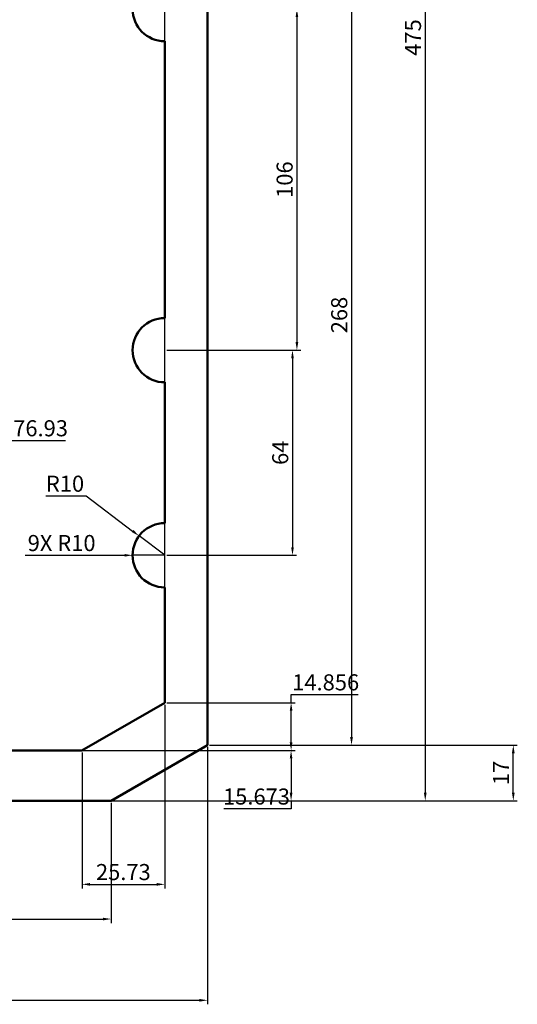
# Model space of a CAD drawing. Units: millimetres. Extents: x 1744 to 2162, y 1763 to 2334.
# Tile 2 of 5: x 2007 to 2162, y 1763 to 2070. Entities that reach past the tile are written whole.
import ezdxf

# ---------------------------------------------------------------- set-up
doc = ezdxf.new("R2010")
doc.units = ezdxf.units.MM
doc.layers.add('M-DIMS', color=2, linetype='Continuous', lineweight=25)
doc.layers.add('M-OUTL', color=7, linetype='Continuous', lineweight=50)
doc.styles.get("Standard").update_dxf_attribs({"font": 'arial.ttf'})
doc.dimstyles.new('ISO-25', dxfattribs={"dimtxt": 5, "dimasz": 2.5, "dimexe": 1.25, "dimexo": 0.625, "dimtad": 1, "dimtoh": 1, "dimdec": 0, "dimtxsty": 'Standard', "dimcen": 2.5, "dimadec": 0, "dimazin": 0, "dimtfac": 1, "dimtdec": 0, "dimtmove": 0, "dimatfit": 3, "dimfxl": 1, "dimarcsym": 0})

# ---------------------------------------------------------------- blocks, each defined once
blk = doc.blocks.new('*D2')
at = {"layer": 'Defpoints', "color": 0, "transparency": 16777216}
for p in [(2029.83, 2301.76), (2035.83, 1826.76), (2133.56, 1826.76)]:
    blk.add_point(p, dxfattribs=at)
at = {"layer": 'M-DIMS', "color": 0, "lineweight": -2, "transparency": 16777216}
for p, q in [((2030.45, 2301.76), (2134.81, 2301.76)), ((2133.56, 2299.26), (2133.56, 1829.26)), ((2036.45, 1826.76), (2134.81, 1826.76))]:
    blk.add_line(p, q, dxfattribs=at)
at = {"layer": 'M-DIMS', "color": 0, "transparency": 16777216}
for points in [[(2133.14, 2299.26), (2133.98, 2299.26), (2133.56, 2301.76)], [(2133.14, 1829.26), (2133.98, 1829.26), (2133.56, 1826.76)]]:
    blk.add_solid(points, dxfattribs=at)
at = {"layer": 'M-DIMS', "color": 0, "transparency": 16777216, "insert": (2130.39, 2064.26), "char_height": 5, "attachment_point": 5, "rotation": 90}
blk.add_mtext('475', dxfattribs=at)
blk = doc.blocks.new('*D4')
at = {"layer": 'Defpoints', "color": 0, "transparency": 16777216}
for p in [(2065.83, 2111.76), (2065.83, 1844.08), (2110.62, 1844.08)]:
    blk.add_point(p, dxfattribs=at)
at = {"layer": 'M-DIMS', "color": 0, "lineweight": -2, "transparency": 16777216}
for p, q in [((2066.45, 2111.76), (2111.87, 2111.76)), ((2110.62, 2109.26), (2110.62, 1846.58)), ((2066.45, 1844.08), (2111.87, 1844.08))]:
    blk.add_line(p, q, dxfattribs=at)
at = {"layer": 'M-DIMS', "color": 0, "transparency": 16777216}
for points in [[(2110.2, 2109.26), (2111.04, 2109.26), (2110.62, 2111.76)], [(2110.2, 1846.58), (2111.04, 1846.58), (2110.62, 1844.08)]]:
    blk.add_solid(points, dxfattribs=at)
at = {"layer": 'M-DIMS', "color": 0, "transparency": 16777216, "insert": (2107.44, 1977.92), "char_height": 5, "attachment_point": 5, "rotation": 90}
blk.add_mtext('268', dxfattribs=at)
blk = doc.blocks.new('*D5')
at = {"layer": 'Defpoints', "color": 0, "transparency": 16777216}
for p in [(2065.83, 1844.08), (2160.95, 1844.08), (2035.83, 1826.76)]:
    blk.add_point(p, dxfattribs=at)
at = {"layer": 'M-DIMS', "color": 0, "lineweight": -2, "transparency": 16777216}
for p, q in [((2066.45, 1844.08), (2162.2, 1844.08)), ((2160.95, 1829.26), (2160.95, 1841.58)), ((2036.45, 1826.76), (2162.2, 1826.76))]:
    blk.add_line(p, q, dxfattribs=at)
at = {"layer": 'M-DIMS', "color": 0, "transparency": 16777216}
for points in [[(2160.53, 1841.58), (2161.37, 1841.58), (2160.95, 1844.08)], [(2160.53, 1829.26), (2161.37, 1829.26), (2160.95, 1826.76)]]:
    blk.add_solid(points, dxfattribs=at)
at = {"layer": 'M-DIMS', "color": 0, "transparency": 16777216, "insert": (2157.81, 1835.42), "char_height": 5, "attachment_point": 5, "rotation": 90}
blk.add_mtext('17', dxfattribs=at)
blk = doc.blocks.new('*D20')
at = {"layer": 'Defpoints', "color": 0, "transparency": 16777216}
for p in [(2044.53, 1909.18), (2052.51, 1903.15)]:
    blk.add_point(p, dxfattribs=at)
at = {"layer": 'M-DIMS', "color": 0, "lineweight": -2, "transparency": 16777216}
for p, q in [((2015.54, 1921.61), (2028.09, 1921.61)), ((2028.09, 1921.61), (2042.53, 1910.69)), ((2052.51, 1903.15), (2044.53, 1909.18))]:
    blk.add_line(p, q, dxfattribs=at)
at = {"layer": 'M-DIMS', "color": 0, "transparency": 16777216}
blk.add_solid([(2042.79, 1911.02), (2042.28, 1910.36), (2044.53, 1909.18)], dxfattribs=at)
at = {"layer": 'M-DIMS', "color": 0, "transparency": 16777216, "insert": (2021.5, 1924.78), "char_height": 5, "attachment_point": 5}
blk.add_mtext('R10', dxfattribs=at)
blk = doc.blocks.new('*D25')
at = {"layer": 'Defpoints', "color": 0, "transparency": 16777216}
for p in [(2052.51, 2073.12), (2052.51, 1966.98), (2093.63, 1966.98)]:
    blk.add_point(p, dxfattribs=at)
at = {"layer": 'M-DIMS', "color": 0, "lineweight": -2, "transparency": 16777216}
for p, q in [((2053.13, 2073.12), (2094.88, 2073.12)), ((2093.63, 2070.62), (2093.63, 1969.48)), ((2053.13, 1966.98), (2094.88, 1966.98))]:
    blk.add_line(p, q, dxfattribs=at)
at = {"layer": 'M-DIMS', "color": 0, "transparency": 16777216}
for points in [[(2093.22, 2070.62), (2094.05, 2070.62), (2093.63, 2073.12)], [(2093.22, 1969.48), (2094.05, 1969.48), (2093.63, 1966.98)]]:
    blk.add_solid(points, dxfattribs=at)
at = {"layer": 'M-DIMS', "color": 0, "transparency": 16777216, "insert": (2090.46, 2020.05), "char_height": 5, "attachment_point": 5, "rotation": 90}
blk.add_mtext('106', dxfattribs=at)
blk = doc.blocks.new('*D26')
at = {"layer": 'Defpoints', "color": 0, "transparency": 16777216}
for p in [(2052.51, 1966.98), (2052.51, 1903.15), (2092.26, 1903.15)]:
    blk.add_point(p, dxfattribs=at)
at = {"layer": 'M-DIMS', "color": 0, "lineweight": -2, "transparency": 16777216}
for p, q in [((2053.13, 1966.98), (2093.51, 1966.98)), ((2092.26, 1964.48), (2092.26, 1905.65)), ((2053.13, 1903.15), (2093.51, 1903.15))]:
    blk.add_line(p, q, dxfattribs=at)
at = {"layer": 'M-DIMS', "color": 0, "transparency": 16777216}
for points in [[(2091.85, 1964.48), (2092.68, 1964.48), (2092.26, 1966.98)], [(2091.85, 1905.65), (2092.68, 1905.65), (2092.26, 1903.15)]]:
    blk.add_solid(points, dxfattribs=at)
at = {"layer": 'M-DIMS', "color": 0, "transparency": 16777216, "insert": (2089.09, 1935.06), "char_height": 5, "attachment_point": 5, "rotation": 90}
blk.add_mtext('64', dxfattribs=at)
blk = doc.blocks.new('*D27')
at = {"layer": 'Defpoints', "color": 0, "transparency": 16777216}
for p in [(1863.15, 1826.76), (2035.83, 1826.76), (2035.83, 1789.97)]:
    blk.add_point(p, dxfattribs=at)
at = {"layer": 'M-DIMS', "color": 0, "lineweight": -2, "transparency": 16777216}
for p, q in [((1863.15, 1826.14), (1863.15, 1788.72)), ((2035.83, 1826.14), (2035.83, 1788.72)), ((1865.65, 1789.97), (2033.33, 1789.97))]:
    blk.add_line(p, q, dxfattribs=at)
at = {"layer": 'M-DIMS', "color": 0, "transparency": 16777216}
for points in [[(1865.65, 1790.38), (1865.65, 1789.55), (1863.15, 1789.97)], [(2033.33, 1790.38), (2033.33, 1789.55), (2035.83, 1789.97)]]:
    blk.add_solid(points, dxfattribs=at)
at = {"layer": 'M-DIMS', "color": 0, "transparency": 16777216, "insert": (1949.49, 1793.15), "char_height": 5, "attachment_point": 5}
blk.add_mtext('173', dxfattribs=at)
blk = doc.blocks.new('*D28')
at = {"layer": 'Defpoints', "color": 0, "transparency": 16777216}
for p in [(1845.83, 1856.76), (2065.83, 1844.08), (2065.83, 1764.69)]:
    blk.add_point(p, dxfattribs=at)
at = {"layer": 'M-DIMS', "color": 0, "lineweight": -2, "transparency": 16777216}
for p, q in [((1845.83, 1856.14), (1845.83, 1763.44)), ((2065.83, 1843.46), (2065.83, 1763.44)), ((1848.33, 1764.69), (2063.33, 1764.69))]:
    blk.add_line(p, q, dxfattribs=at)
at = {"layer": 'M-DIMS', "color": 0, "transparency": 16777216}
for points in [[(1848.33, 1765.1), (1848.33, 1764.27), (1845.83, 1764.69)], [(2063.33, 1765.1), (2063.33, 1764.27), (2065.83, 1764.69)]]:
    blk.add_solid(points, dxfattribs=at)
at = {"layer": 'M-DIMS', "color": 0, "transparency": 16777216, "insert": (1955.83, 1767.86), "char_height": 5, "attachment_point": 5}
blk.add_mtext('220', dxfattribs=at)
blk = doc.blocks.new('*D29')
at = {"layer": 'Defpoints', "color": 0, "transparency": 16777216}
for p in [(2052.51, 2327.76), (2052.51, 1966.98), (1937.15, 1938.72)]:
    blk.add_point(p, dxfattribs=at)
at = {"layer": 'M-DIMS', "color": 0, "lineweight": -2, "transparency": 16777216}
for p, q in [((1937.15, 1939.34), (1937.15, 2329.01)), ((2052.51, 1967.6), (2052.51, 2329.01)), ((1939.65, 2327.76), (2050.01, 2327.76))]:
    blk.add_line(p, q, dxfattribs=at)
at = {"layer": 'M-DIMS', "color": 0, "transparency": 16777216}
for points in [[(1939.65, 2328.18), (1939.65, 2327.34), (1937.15, 2327.76)], [(2050.01, 2328.18), (2050.01, 2327.34), (2052.51, 2327.76)]]:
    blk.add_solid(points, dxfattribs=at)
at = {"layer": 'M-DIMS', "color": 0, "transparency": 16777216, "insert": (1994.83, 2330.94), "char_height": 5, "attachment_point": 5}
blk.add_mtext('115.35', dxfattribs=at)
blk = doc.blocks.new('*D46')
at = {"layer": 'Defpoints', "color": 0, "transparency": 16777216}
for p in [(2052.51, 2327.76), (1861.12, 1859.18), (2052.51, 1857.29)]:
    blk.add_point(p, dxfattribs=at)
at = {"layer": 'M-DIMS', "color": 0, "lineweight": -2, "transparency": 16777216}
for p, q in [((1861.12, 1859.81), (1861.12, 2329.01)), ((2052.51, 1857.91), (2052.51, 2329.01)), ((1863.62, 2327.76), (2050.01, 2327.76))]:
    blk.add_line(p, q, dxfattribs=at)
at = {"layer": 'M-DIMS', "color": 0, "transparency": 16777216}
for points in [[(1863.62, 2328.18), (1863.62, 2327.34), (1861.12, 2327.76)], [(2050.01, 2328.18), (2050.01, 2327.34), (2052.51, 2327.76)]]:
    blk.add_solid(points, dxfattribs=at)
at = {"layer": 'M-DIMS', "color": 0, "transparency": 16777216, "insert": (1956.82, 2330.94), "char_height": 5, "attachment_point": 5}
blk.add_mtext('191.4', dxfattribs=at)
blk = doc.blocks.new('*D49')
at = {"layer": 'Defpoints', "color": 0, "transparency": 16777216}
for p in [(1870.79, 1842.43), (1863.15, 1826.76), (2091.83, 1826.76)]:
    blk.add_point(p, dxfattribs=at)
at = {"layer": 'M-DIMS', "color": 0, "lineweight": -2, "transparency": 16777216}
for p, q in [((1871.42, 1842.43), (2093.08, 1842.43)), ((2091.83, 1839.93), (2091.83, 1829.26)), ((1863.77, 1826.76), (2093.08, 1826.76)), ((2091.83, 1826.76), (2091.83, 1824.26)), ((2091.83, 1824.26), (2070.91, 1824.26))]:
    blk.add_line(p, q, dxfattribs=at)
at = {"layer": 'M-DIMS', "color": 0, "transparency": 16777216}
for points in [[(2091.41, 1839.93), (2092.24, 1839.93), (2091.83, 1842.43)], [(2091.41, 1829.26), (2092.24, 1829.26), (2091.83, 1826.76)]]:
    blk.add_solid(points, dxfattribs=at)
at = {"layer": 'M-DIMS', "color": 0, "transparency": 16777216, "insert": (2081.06, 1827.44), "char_height": 5, "attachment_point": 5}
blk.add_mtext('15.673', dxfattribs=at)
blk = doc.blocks.new('*D65')
at = {"layer": 'Defpoints', "color": 0, "transparency": 16777216}
for p in [(2052.51, 1857.29), (2091.83, 1857.29), (2026.78, 1842.43)]:
    blk.add_point(p, dxfattribs=at)
at = {"layer": 'M-DIMS', "color": 0, "lineweight": -2, "transparency": 16777216}
for p, q in [((2091.83, 1857.29), (2091.83, 1859.79)), ((2091.83, 1859.79), (2112.73, 1859.79)), ((2053.13, 1857.29), (2093.08, 1857.29)), ((2091.83, 1844.93), (2091.83, 1854.79)), ((2027.4, 1842.43), (2093.08, 1842.43))]:
    blk.add_line(p, q, dxfattribs=at)
at = {"layer": 'M-DIMS', "color": 0, "transparency": 16777216}
for points in [[(2091.41, 1854.79), (2092.24, 1854.79), (2091.83, 1857.29)], [(2091.41, 1844.93), (2092.24, 1844.93), (2091.83, 1842.43)]]:
    blk.add_solid(points, dxfattribs=at)
at = {"layer": 'M-DIMS', "color": 0, "transparency": 16777216, "insert": (2102.59, 1862.97), "char_height": 5, "attachment_point": 5}
blk.add_mtext('14.856', dxfattribs=at)
blk = doc.blocks.new('*D66')
at = {"layer": 'Defpoints', "color": 0, "transparency": 16777216}
for p in [(2052.51, 1857.29), (2026.78, 1842.43), (2052.51, 1800.76)]:
    blk.add_point(p, dxfattribs=at)
at = {"layer": 'M-DIMS', "color": 0, "lineweight": -2, "transparency": 16777216}
for p, q in [((2052.51, 1856.66), (2052.51, 1799.51)), ((2026.78, 1841.81), (2026.78, 1799.51)), ((2029.28, 1800.76), (2050.01, 1800.76))]:
    blk.add_line(p, q, dxfattribs=at)
at = {"layer": 'M-DIMS', "color": 0, "transparency": 16777216}
for points in [[(2029.28, 1801.18), (2029.28, 1800.34), (2026.78, 1800.76)], [(2050.01, 1801.18), (2050.01, 1800.34), (2052.51, 1800.76)]]:
    blk.add_solid(points, dxfattribs=at)
at = {"layer": 'M-DIMS', "color": 0, "transparency": 16777216, "insert": (2039.64, 1803.94), "char_height": 5, "attachment_point": 5}
blk.add_mtext('25.73', dxfattribs=at)
blk = doc.blocks.new('*D78')
at = {"layer": 'Defpoints', "color": 0, "transparency": 16777216}
for p in [(1898.69, 1938.72), (1975.62, 1938.72)]:
    blk.add_point(p, dxfattribs=at)
at = {"layer": 'M-DIMS', "color": 0, "lineweight": -2, "transparency": 16777216}
for p, q in [((1896.19, 1938.72), (1893.69, 1938.72)), ((1898.69, 1938.72), (1975.62, 1938.72)), ((1998.7, 1938.72), (1978.12, 1938.72)), ((2021.64, 1938.72), (1998.7, 1938.72))]:
    blk.add_line(p, q, dxfattribs=at)
at = {"layer": 'M-DIMS', "color": 0, "transparency": 16777216}
for points in [[(1896.19, 1939.13), (1896.19, 1938.3), (1898.69, 1938.72)], [(1978.12, 1939.13), (1978.12, 1938.3), (1975.62, 1938.72)]]:
    blk.add_solid(points, dxfattribs=at)
at = {"layer": 'M-DIMS', "color": 0, "transparency": 16777216, "insert": (2010.48, 1942.03), "char_height": 5, "attachment_point": 5}
blk.add_mtext('∅76.93', dxfattribs=at)
blk = doc.blocks.new('*D88')
at = {"layer": 'Defpoints', "color": 0, "transparency": 16777216}
for p in [(2042.51, 1903.15), (2052.51, 1903.15)]:
    blk.add_point(p, dxfattribs=at)
at = {"layer": 'M-DIMS', "color": 0, "lineweight": -2, "transparency": 16777216}
for p, q in [((2009.1, 1903.15), (2032.4, 1903.15)), ((2032.4, 1903.15), (2040.01, 1903.15)), ((2052.51, 1903.15), (2042.51, 1903.15))]:
    blk.add_line(p, q, dxfattribs=at)
at = {"layer": 'M-DIMS', "color": 0, "transparency": 16777216}
blk.add_solid([(2040.01, 1903.57), (2040.01, 1902.73), (2042.51, 1903.15)], dxfattribs=at)
at = {"layer": 'M-DIMS', "color": 0, "transparency": 16777216, "insert": (2020.44, 1906.32), "char_height": 5, "attachment_point": 5}
blk.add_mtext('9X R10', dxfattribs=at)

msp = doc.modelspace()

# ---------------------------------------------------------------- linework, layer by layer
at = {"layer": 'M-OUTL'}
for p, q in [((2065.8255, 1844.0809), (2065.8255, 2111.7604)), ((2052.5068, 1976.9753), (2052.5068, 2063.1218)), ((2052.5068, 1913.1533), (2052.5068, 1956.9753)), ((2052.5068, 1857.2889), (2052.5068, 1893.1533)), ((2026.7766, 1842.4335), (2052.5068, 1857.2889)), ((1870.7949, 1842.4331), (2026.7759, 1842.4331)), ((2026.7766, 1842.4335), (2026.7759, 1842.4331)), ((2035.8255, 1826.7604), (2065.8255, 1844.0809)), ((1863.146, 1826.7604), (2035.8255, 1826.7604))]:
    msp.add_line(p, q, dxfattribs=at)
for centre in [(2052.5068, 2073.1218), (2052.5068, 1966.9753), (2052.5068, 1903.1533)]:
    msp.add_arc(centre, 10, 90, 270, dxfattribs=at)

# ---------------------------------------------------------------- dimensions: what is measured, and where the dimension line sits
at = {"layer": 'M-DIMS'}
for base, p1, p2, override, picture, middle in [((2052.5068, 2327.7604), (1861.1237, 1859.184), (2052.5068, 1857.2889), {"dimdec": 1, "dimlfac": 1, "dimrnd": 0, "dimzin": 0, "dimdsep": 46, "dimlunit": 2}, '*D46', (1956.8153, 2330.9382)), ((2052.5068, 2327.7604), (1937.1543, 1938.7171), (2052.5068, 1966.9753), {"dimdec": 2, "dimlfac": 1, "dimrnd": 0, "dimzin": 0, "dimdsep": 46, "dimlunit": 2}, '*D29', (1994.8306, 2330.9399)), ((2065.8255, 1764.685), (1845.8255, 1856.7604), (2065.8255, 1844.0809), {"dimclrd": 0, "dimclre": 0, "dimclrt": 0}, '*D28', (1955.8255, 1767.8629)), ((2052.5068, 1800.7604), (2026.7759, 1842.4331), (2052.5068, 1857.2889), {"dimdec": 2, "dimlfac": 1, "dimrnd": 0, "dimzin": 0, "dimdsep": 46, "dimlunit": 2}, '*D66', (2039.6413, 1803.9399)), ((2035.8255, 1789.9672), (1863.146, 1826.7604), (2035.8255, 1826.7604), {"dimclrd": 0, "dimclre": 0, "dimclrt": 0}, '*D27', (1949.4857, 1793.1468))]:
    dim = msp.add_linear_dim(base=base, p1=p1, p2=p2, dimstyle='ISO-25', override=override, dxfattribs=at)
    dim.commit()
    dim.dimension.update_dxf_attribs({"geometry": picture, "text_midpoint": middle})
for base, p1, p2, override, picture, middle in [((2133.5602, 1826.7604), (2029.8255, 2301.7604), (2035.8255, 1826.7604), {"dimclrd": 0, "dimclre": 0, "dimclrt": 0}, '*D2', (2130.3925, 2064.2604)), ((2110.6209, 1844.0809), (2065.8255, 2111.7604), (2065.8255, 1844.0809), {"dimclrd": 0, "dimclre": 0, "dimclrt": 0}, '*D4', (2107.4431, 1977.9206)), ((2093.6333, 1966.9753), (2052.5068, 2073.1218), (2052.5068, 1966.9753), {"dimclrd": 0, "dimclre": 0, "dimclrt": 0}, '*D25', (2090.4554, 2020.0486)), ((2092.2638, 1903.1533), (2052.5068, 1966.9753), (2052.5068, 1903.1533), {"dimclrd": 0, "dimclre": 0, "dimclrt": 0}, '*D26', (2089.086, 1935.0643)), ((2091.8255, 1857.2889), (2026.7759, 1842.4331), (2052.5068, 1857.2889), {"dimdec": 3, "dimlfac": 1, "dimrnd": 0, "dimzin": 0, "dimdsep": 46, "dimlunit": 2}, '*D65', (2102.592, 1862.9667)), ((2091.8255, 1826.7604), (1870.7949, 1842.4331), (1863.146, 1826.7604), {"dimdec": 3, "dimlfac": 1, "dimrnd": 0, "dimzin": 0, "dimdsep": 46, "dimlunit": 2}, '*D49', (2081.0572, 1827.4399)), ((2160.949, 1844.0809), (2035.8255, 1826.7604), (2065.8255, 1844.0809), {"dimclrd": 0, "dimclre": 0, "dimclrt": 0}, '*D5', (2157.8138, 1835.4206))]:
    dim = msp.add_linear_dim(base=base, p1=p1, p2=p2, angle=90, dimstyle='ISO-25', override=override, dxfattribs=at)
    dim.commit()
    dim.dimension.update_dxf_attribs({"geometry": picture, "text_midpoint": middle})
dim = msp.add_diameter_dim_2p(p1=(1898.6872, 1938.7172), p2=(1975.6215, 1938.717), dimstyle='ISO-25', override={"dimdec": 2, "dimlfac": 1, "dimrnd": 0, "dimzin": 0, "dimdsep": 46, "dimlunit": 2}, dxfattribs=at)
dim.commit()
dim.dimension.update_dxf_attribs({"geometry": '*D78', "text_midpoint": (1998.7017, 1938.717), "dimtype": 163})
dim = msp.add_radius_dim(center=(2052.5068, 1903.1533), mpoint=(2044.529, 1909.1828), dimstyle='ISO-25', override={"dimclrd": 0, "dimclre": 0, "dimclrt": 0}, dxfattribs=at)
dim.commit()
dim.dimension.update_dxf_attribs({"geometry": '*D20', "text_midpoint": (2021.503, 1921.6051), "dimtype": 164})
dim = msp.add_radius_dim(center=(2052.5068, 1903.1533), mpoint=(2042.5068, 1903.15), text='9X <>', dimstyle='ISO-25', override={"dimdec": 0, "dimlfac": 1, "dimrnd": 0, "dimzin": 0, "dimdsep": 46, "dimlunit": 2}, dxfattribs=at)
dim.commit()
dim.dimension.update_dxf_attribs({"geometry": '*D88', "text_midpoint": (2020.4391, 1906.3246)})

doc.saveas('drawing.dxf')
